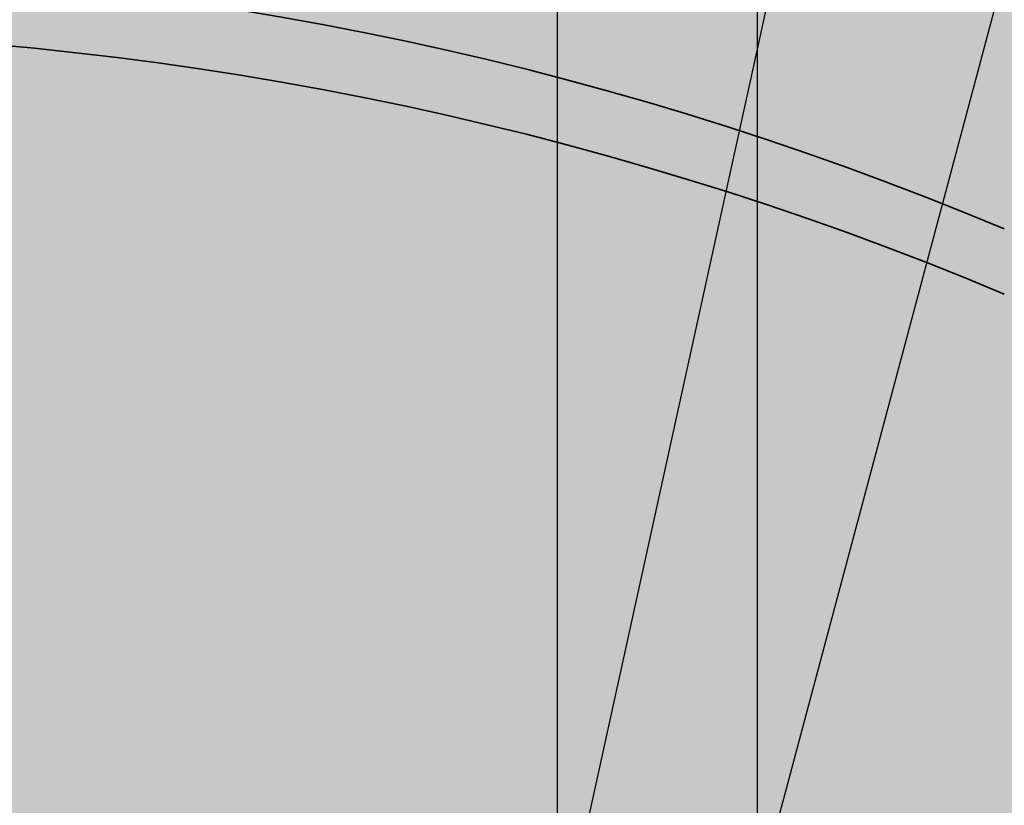
# Model space of a CAD drawing. Units: millimetres. Extents: x 130 to 1021, y 147 to 699.
# Tile 24 of 40: x 442 to 487, y 440 to 477. Entities that reach past the tile are written whole.
import ezdxf

# ---------------------------------------------------------------- set-up
doc = ezdxf.new("R2010")
doc.units = ezdxf.units.MM
doc.header["$MEASUREMENT"] = 0
for name, color, linetype, lineweight in [('A-ANNO-DIMS', 2, 'Continuous', 18), ('A-ELEV', 7, 'Continuous', 35), ('A-ELEV-PATT', 9, 'Continuous', 13)]:
    doc.layers.add(name, color=color, linetype=linetype, lineweight=lineweight)
doc.styles.get("Standard").update_dxf_attribs({"font": 'arial.ttf'})
doc.dimstyles.get("Standard").update_dxf_attribs({"dimtxt": 20, "dimasz": 10, "dimexe": 10, "dimexo": 10, "dimgap": 5, "dimtad": 0, "dimtih": 1, "dimtoh": 1, "dimdec": 0, "dimzin": 0, "dimdsep": 46, "dimtxsty": 'Standard', "dimcen": 5, "dimadec": 0, "dimazin": 0, "dimtfac": 1, "dimtdec": 0, "dimtofl": 0, "dimtmove": 0, "dimatfit": 3, "dimfxl": 1, "dimtolj": 1, "dimtzin": 0, "dimarcsym": 0})

# ---------------------------------------------------------------- blocks, each defined once
blk = doc.blocks.new('*D11')
at = {"layer": 'A-ANNO-DIMS', "color": 0, "lineweight": -2, "transparency": 16777216}
for p, q in [((737.374, 648.699), (737.374, 149.739)), ((299.374, 566.947), (299.374, 149.739)), ((309.374, 159.739), (490.857, 159.739)), ((727.374, 159.739), (545.891, 159.739))]:
    blk.add_line(p, q, dxfattribs=at)
at = {"layer": 'A-ANNO-DIMS', "color": 0, "transparency": 16777216}
for points in [[(309.374, 161.406), (309.374, 158.073), (299.374, 159.739)], [(727.374, 161.406), (727.374, 158.073), (737.374, 159.739)]]:
    blk.add_solid(points, dxfattribs=at)
at = {"layer": 'Defpoints', "color": 0, "transparency": 16777216}
for p in [(737.374, 658.699), (299.374, 576.947), (737.374, 159.739)]:
    blk.add_point(p, dxfattribs=at)
at = {"layer": 'A-ANNO-DIMS', "color": 0, "transparency": 16777216, "insert": (518.374, 159.739), "char_height": 20, "attachment_point": 5}
blk.add_mtext('\\A1;438', dxfattribs=at)
blk = doc.blocks.new('*D12')
at = {"layer": 'A-ANNO-DIMS', "color": 0, "lineweight": -2, "transparency": 16777216}
for p, q in [((477.374, 661.947), (265.074, 661.947)), ((275.074, 651.947), (275.074, 438.205)), ((275.074, 194.039), (275.074, 407.782)), ((357.163, 184.039), (265.074, 184.039))]:
    blk.add_line(p, q, dxfattribs=at)
at = {"layer": 'A-ANNO-DIMS', "color": 0, "transparency": 16777216}
for points in [[(273.407, 651.947), (276.74, 651.947), (275.074, 661.947)], [(273.407, 194.039), (276.74, 194.039), (275.074, 184.039)]]:
    blk.add_solid(points, dxfattribs=at)
at = {"layer": 'Defpoints', "color": 0, "transparency": 16777216}
for p in [(275.074, 661.947), (487.374, 661.947), (367.163, 184.039)]:
    blk.add_point(p, dxfattribs=at)
at = {"layer": 'A-ANNO-DIMS', "color": 0, "transparency": 16777216, "insert": (275.074, 422.993), "char_height": 20, "attachment_point": 5}
blk.add_mtext('\\A1;477.9', dxfattribs=at)
blk = doc.blocks.new('*D16')
at = {"layer": 'A-ANNO-DIMS', "color": 0, "lineweight": -2, "transparency": 16777216}
for p, q in [((357.941, 411.947), (357.941, 696.247)), ((363.922, 579.884), (363.922, 696.247)), ((347.941, 686.247), (337.941, 686.247)), ((373.922, 686.247), (383.922, 686.247))]:
    blk.add_line(p, q, dxfattribs=at)
at = {"layer": 'A-ANNO-DIMS', "color": 0, "transparency": 16777216}
for points in [[(347.941, 687.914), (347.941, 684.581), (357.941, 686.247)], [(373.922, 687.914), (373.922, 684.581), (363.922, 686.247)]]:
    blk.add_solid(points, dxfattribs=at)
at = {"layer": 'Defpoints', "color": 0, "transparency": 16777216}
for p in [(363.922, 686.247), (363.922, 569.884), (357.941, 401.947)]:
    blk.add_point(p, dxfattribs=at)
at = {"layer": 'A-ANNO-DIMS', "color": 0, "transparency": 16777216, "insert": (420.737, 686.247), "char_height": 20, "attachment_point": 5}
blk.add_mtext('\\A1;5.981', dxfattribs=at)
blk = doc.blocks.new('*D18')
at = {"layer": 'A-ANNO-DIMS', "color": 0, "lineweight": -2, "transparency": 16777216}
for p, q in [((375.85, 490.216), (375.85, 696.247)), ((382.374, 388.947), (382.374, 696.247)), ((365.85, 686.247), (355.85, 686.247)), ((392.374, 686.247), (402.374, 686.247))]:
    blk.add_line(p, q, dxfattribs=at)
at = {"layer": 'A-ANNO-DIMS', "color": 0, "transparency": 16777216}
for points in [[(365.85, 687.914), (365.85, 684.581), (375.85, 686.247)], [(392.374, 687.914), (392.374, 684.581), (382.374, 686.247)]]:
    blk.add_solid(points, dxfattribs=at)
at = {"layer": 'Defpoints', "color": 0, "transparency": 16777216}
for p in [(382.374, 686.247), (375.85, 480.216), (382.374, 378.947)]:
    blk.add_point(p, dxfattribs=at)
at = {"layer": 'A-ANNO-DIMS', "color": 0, "transparency": 16777216, "insert": (441.132, 686.247), "char_height": 20, "attachment_point": 5}
blk.add_mtext('\\A1;6.524', dxfattribs=at)
blk = doc.blocks.new('*D19')
at = {"layer": 'A-ANNO-DIMS', "color": 0, "lineweight": -2, "transparency": 16777216}
for p, q in [((382.374, 388.947), (382.374, 696.247)), ((414.652, 510.881), (414.652, 696.247)), ((392.374, 686.247), (404.652, 686.247)), ((414.652, 686.247), (424.652, 686.247))]:
    blk.add_line(p, q, dxfattribs=at)
at = {"layer": 'A-ANNO-DIMS', "color": 0, "transparency": 16777216}
for points in [[(392.374, 687.914), (392.374, 684.581), (382.374, 686.247)], [(404.652, 687.914), (404.652, 684.581), (414.652, 686.247)]]:
    blk.add_solid(points, dxfattribs=at)
at = {"layer": 'Defpoints', "color": 0, "transparency": 16777216}
for p in [(414.652, 686.247), (414.652, 500.881), (382.374, 378.947)]:
    blk.add_point(p, dxfattribs=at)
at = {"layer": 'A-ANNO-DIMS', "color": 0, "transparency": 16777216, "insert": (463.411, 686.247), "char_height": 20, "attachment_point": 5}
blk.add_mtext('\\A1;32.28', dxfattribs=at)
blk = doc.blocks.new('*D20')
at = {"layer": 'A-ANNO-DIMS', "color": 0, "lineweight": -2, "transparency": 16777216}
for p, q in [((414.652, 510.881), (414.652, 696.247)), ((432.374, 388.947), (432.374, 696.247)), ((404.652, 686.247), (394.652, 686.247)), ((442.374, 686.247), (452.374, 686.247))]:
    blk.add_line(p, q, dxfattribs=at)
at = {"layer": 'A-ANNO-DIMS', "color": 0, "transparency": 16777216}
for points in [[(404.652, 687.914), (404.652, 684.581), (414.652, 686.247)], [(442.374, 687.914), (442.374, 684.581), (432.374, 686.247)]]:
    blk.add_solid(points, dxfattribs=at)
at = {"layer": 'Defpoints', "color": 0, "transparency": 16777216}
for p in [(432.374, 686.247), (414.652, 500.881), (432.374, 378.947)]:
    blk.add_point(p, dxfattribs=at)
at = {"layer": 'A-ANNO-DIMS', "color": 0, "transparency": 16777216, "insert": (490.075, 686.247), "char_height": 20, "attachment_point": 5}
blk.add_mtext('\\A1;17.72', dxfattribs=at)
blk = doc.blocks.new('*D21')
at = {"layer": 'A-ANNO-DIMS', "color": 0, "lineweight": -2, "transparency": 16777216}
for p, q in [((432.374, 388.947), (432.374, 696.247)), ((447.374, 656.947), (447.374, 696.247)), ((422.374, 686.247), (412.374, 686.247)), ((457.374, 686.247), (467.374, 686.247))]:
    blk.add_line(p, q, dxfattribs=at)
at = {"layer": 'A-ANNO-DIMS', "color": 0, "transparency": 16777216}
for points in [[(422.374, 687.914), (422.374, 684.581), (432.374, 686.247)], [(457.374, 687.914), (457.374, 684.581), (447.374, 686.247)]]:
    blk.add_solid(points, dxfattribs=at)
at = {"layer": 'Defpoints', "color": 0, "transparency": 16777216}
for p in [(447.374, 686.247), (447.374, 646.947), (432.374, 378.947)]:
    blk.add_point(p, dxfattribs=at)
at = {"layer": 'A-ANNO-DIMS', "color": 0, "transparency": 16777216, "insert": (485.832, 686.247), "char_height": 20, "attachment_point": 5}
blk.add_mtext('\\A1;15', dxfattribs=at)
blk = doc.blocks.new('*D22')
at = {"layer": 'A-ANNO-DIMS', "color": 0, "lineweight": -2, "transparency": 16777216}
for p, q in [((447.374, 656.947), (447.374, 696.247)), ((466.767, 403.947), (466.767, 696.247)), ((437.374, 686.247), (427.374, 686.247)), ((476.767, 686.247), (486.767, 686.247))]:
    blk.add_line(p, q, dxfattribs=at)
at = {"layer": 'A-ANNO-DIMS', "color": 0, "transparency": 16777216}
for points in [[(437.374, 687.914), (437.374, 684.581), (447.374, 686.247)], [(476.767, 687.914), (476.767, 684.581), (466.767, 686.247)]]:
    blk.add_solid(points, dxfattribs=at)
at = {"layer": 'Defpoints', "color": 0, "transparency": 16777216}
for p in [(466.767, 686.247), (447.374, 646.947), (466.767, 393.947)]:
    blk.add_point(p, dxfattribs=at)
at = {"layer": 'A-ANNO-DIMS', "color": 0, "transparency": 16777216, "insert": (532.34, 686.247), "char_height": 20, "attachment_point": 5}
blk.add_mtext('\\A1;19.393', dxfattribs=at)
blk = doc.blocks.new('*D23')
at = {"layer": 'A-ANNO-DIMS', "color": 0, "lineweight": -2, "transparency": 16777216}
for p, q in [((466.767, 403.947), (466.767, 696.247)), ((475.988, 209.039), (475.988, 696.247)), ((456.767, 686.247), (446.767, 686.247)), ((485.988, 686.247), (495.988, 686.247))]:
    blk.add_line(p, q, dxfattribs=at)
at = {"layer": 'A-ANNO-DIMS', "color": 0, "transparency": 16777216}
for points in [[(456.767, 687.914), (456.767, 684.581), (466.767, 686.247)], [(485.988, 687.914), (485.988, 684.581), (475.988, 686.247)]]:
    blk.add_solid(points, dxfattribs=at)
at = {"layer": 'Defpoints', "color": 0, "transparency": 16777216}
for p in [(475.988, 686.247), (466.767, 393.947), (475.988, 199.039)]:
    blk.add_point(p, dxfattribs=at)
at = {"layer": 'A-ANNO-DIMS', "color": 0, "transparency": 16777216, "insert": (534.631, 686.247), "char_height": 20, "attachment_point": 5}
blk.add_mtext('\\A1;9.222', dxfattribs=at)
blk = doc.blocks.new('*D24')
at = {"layer": 'A-ANNO-DIMS', "color": 0, "lineweight": -2, "transparency": 16777216}
for p, q in [((475.988, 209.039), (475.988, 696.247)), ((487.374, 671.947), (487.374, 696.247)), ((465.988, 686.247), (455.988, 686.247)), ((497.374, 686.247), (507.374, 686.247))]:
    blk.add_line(p, q, dxfattribs=at)
at = {"layer": 'A-ANNO-DIMS', "color": 0, "transparency": 16777216}
for points in [[(465.988, 687.914), (465.988, 684.581), (475.988, 686.247)], [(497.374, 687.914), (497.374, 684.581), (487.374, 686.247)]]:
    blk.add_solid(points, dxfattribs=at)
at = {"layer": 'Defpoints', "color": 0, "transparency": 16777216}
for p in [(487.374, 686.247), (487.374, 661.947), (475.988, 199.039)]:
    blk.add_point(p, dxfattribs=at)
at = {"layer": 'A-ANNO-DIMS', "color": 0, "transparency": 16777216, "insert": (553.022, 686.247), "char_height": 20, "attachment_point": 5}
blk.add_mtext('\\A1;11.385', dxfattribs=at)
blk = doc.blocks.new('*D64')
at = {"layer": 'A-ANNO-DIMS', "color": 0, "lineweight": -2, "transparency": 16777216}
for p, q in [((502.049, 450.926), (502.049, 460.926)), ((497.049, 455.926), (507.049, 455.926)), ((363.96, 263.061), (409.922, 327.255)), ((353.96, 263.061), (363.96, 263.061))]:
    blk.add_line(p, q, dxfattribs=at)
at = {"layer": 'A-ANNO-DIMS', "color": 0, "transparency": 16777216}
blk.add_solid([(408.567, 328.225), (411.277, 326.284), (415.743, 335.385)], dxfattribs=at)
at = {"layer": 'Defpoints', "color": 0, "transparency": 16777216}
for p in [(502.049, 455.926), (415.743, 335.385)]:
    blk.add_point(p, dxfattribs=at)
at = {"layer": 'A-ANNO-DIMS', "color": 0, "transparency": 16777216, "insert": (297.8, 263.061), "char_height": 20, "attachment_point": 5}
blk.add_mtext('\\A1;R148.25', dxfattribs=at)
blk = doc.blocks.new('*D65')
at = {"layer": 'A-ANNO-DIMS', "color": 0, "lineweight": -2, "transparency": 16777216}
for p, q in [((495.463, 509.127), (472.508, 423.108)), ((505.463, 509.127), (495.463, 509.127)), ((427.374, 248.979), (427.374, 258.979)), ((422.374, 253.979), (432.374, 253.979))]:
    blk.add_line(p, q, dxfattribs=at)
at = {"layer": 'A-ANNO-DIMS', "color": 0, "transparency": 16777216}
blk.add_solid([(470.898, 423.538), (474.118, 422.679), (469.93, 413.447)], dxfattribs=at)
at = {"layer": 'Defpoints', "color": 0, "transparency": 16777216}
for p in [(469.93, 413.447), (427.374, 253.979)]:
    blk.add_point(p, dxfattribs=at)
at = {"layer": 'A-ANNO-DIMS', "color": 0, "transparency": 16777216, "insert": (561.623, 509.127), "char_height": 20, "attachment_point": 5}
blk.add_mtext('\\A1;R165.05', dxfattribs=at)
blk = doc.blocks.new('*D67')
at = {"layer": 'A-ANNO-DIMS', "color": 0, "lineweight": -2, "transparency": 16777216}
for p, q in [((479.756, 492.431), (462.144, 412.223)), ((489.756, 492.431), (479.756, 492.431)), ((427.07, 247.496), (427.07, 257.496)), ((422.07, 252.496), (432.07, 252.496))]:
    blk.add_line(p, q, dxfattribs=at)
at = {"layer": 'A-ANNO-DIMS', "color": 0, "transparency": 16777216}
blk.add_solid([(460.516, 412.58), (463.772, 411.865), (459.999, 402.455)], dxfattribs=at)
at = {"layer": 'Defpoints', "color": 0, "transparency": 16777216}
for p in [(459.999, 402.455), (427.07, 252.496)]:
    blk.add_point(p, dxfattribs=at)
at = {"layer": 'A-ANNO-DIMS', "color": 0, "transparency": 16777216, "insert": (545.841, 492.431), "char_height": 20, "attachment_point": 5}
blk.add_mtext('\\A1;R153.53', dxfattribs=at)
blk = doc.blocks.new('*D69')
at = {"layer": 'A-ANNO-DIMS', "color": 0, "lineweight": -2, "transparency": 16777216}
for p, q in [((507.746, 572.261), (483.091, 501.813)), ((517.746, 572.261), (507.746, 572.261)), ((433.191, 354.23), (433.191, 364.23)), ((428.191, 359.23), (438.191, 359.23))]:
    blk.add_line(p, q, dxfattribs=at)
at = {"layer": 'A-ANNO-DIMS', "color": 0, "transparency": 16777216}
blk.add_solid([(481.518, 502.363), (484.664, 501.262), (479.788, 492.374)], dxfattribs=at)
at = {"layer": 'Defpoints', "color": 0, "transparency": 16777216}
for p in [(479.788, 492.374), (433.191, 359.23)]:
    blk.add_point(p, dxfattribs=at)
at = {"layer": 'A-ANNO-DIMS', "color": 0, "transparency": 16777216, "insert": (573.824, 572.261), "char_height": 20, "attachment_point": 5}
blk.add_mtext('\\A1;R141.06', dxfattribs=at)
blk = doc.blocks.new('*D71')
at = {"layer": 'A-ANNO-DIMS', "color": 0, "lineweight": -2, "transparency": 16777216}
for p, q in [((492.108, 581.609), (472.542, 512.666)), ((502.108, 581.609), (492.108, 581.609)), ((432.65, 367.109), (432.65, 377.109)), ((427.65, 372.109), (437.65, 372.109))]:
    blk.add_line(p, q, dxfattribs=at)
at = {"layer": 'A-ANNO-DIMS', "color": 0, "transparency": 16777216}
blk.add_solid([(470.938, 513.121), (474.145, 512.211), (469.812, 503.046)], dxfattribs=at)
at = {"layer": 'Defpoints', "color": 0, "transparency": 16777216}
for p in [(469.812, 503.046), (432.65, 372.109)]:
    blk.add_point(p, dxfattribs=at)
at = {"layer": 'A-ANNO-DIMS', "color": 0, "transparency": 16777216, "insert": (548.493, 581.609), "char_height": 20, "attachment_point": 5}
blk.add_mtext('\\A1;R136.1', dxfattribs=at)
blk = doc.blocks.new('*D72')
at = {"layer": 'A-ANNO-DIMS', "color": 0, "lineweight": -2, "transparency": 16777216}
for p, q in [((460.658, 573.64), (451.279, 503.49)), ((470.658, 573.64), (460.658, 573.64)), ((432.115, 355.142), (432.115, 365.142)), ((427.115, 360.142), (437.115, 360.142))]:
    blk.add_line(p, q, dxfattribs=at)
at = {"layer": 'A-ANNO-DIMS', "color": 0, "transparency": 16777216}
blk.add_solid([(449.628, 503.711), (452.931, 503.27), (449.954, 493.579)], dxfattribs=at)
at = {"layer": 'Defpoints', "color": 0, "transparency": 16777216}
for p in [(449.954, 493.579), (432.115, 360.142)]:
    blk.add_point(p, dxfattribs=at)
at = {"layer": 'A-ANNO-DIMS', "color": 0, "transparency": 16777216, "insert": (526.64, 573.64), "char_height": 20, "attachment_point": 5}
blk.add_mtext('\\A1;R134.62', dxfattribs=at)

msp = doc.modelspace()

# ---------------------------------------------------------------- hatches: boundary and pattern name
at = {"layer": 'A-ELEV-PATT'}
h = msp.add_hatch(color=256, dxfattribs=at)
h.dxf.hatch_style = 1
h.paths.add_polyline_path([(737.3738, 658.6988, 0.0135961), (632.4019, 661.9473), (607.3738, 661.9473), (487.3738, 661.9473), (487.3738, 649.9473), (607.3738, 649.9473), (632.3794, 649.9473, -0.0136841), (737.3738, 646.6784)])
h.paths.add_polyline_path([(732.3738, 643.9599, 0.0130529), (632.3738, 646.9473), (607.3738, 646.9473), (487.3738, 646.9473), (487.3738, 596.9473), (632.3738, 596.9473, -0.0130529), (732.3738, 593.9599)])
h.paths.add_polyline_path([(737.3738, 593.6732, 0.0137063), (632.3738, 596.9473), (487.3738, 596.9473), (487.3738, 586.9473), (632.355, 586.9473, -0.0137808), (737.3738, 583.6559)])
h.paths.add_polyline_path([(447.3738, 646.9473), (307.3738, 646.9473), (302.3738, 646.9473), (302.3738, 634.9473), (447.3738, 634.9473)])
h.paths.add_polyline_path([(447.3738, 631.9473), (307.3738, 631.9473), (307.3738, 586.9473), (447.3738, 586.9473)])
h.paths.add_polyline_path([(447.3738, 586.9473), (307.3738, 586.9473), (302.3738, 586.9473), (302.3738, 576.9473), (447.3738, 576.9473)])
h.paths.add_polyline_path([(447.3738, 573.9473), (367.3738, 573.9473), (367.3738, 539.9473), (447.3738, 539.9473)])
h.paths.add_polyline_path([(447.3738, 537.9473), (367.3738, 537.9473), (367.3738, 507.9473), (400.392, 507.4253, -0.001728), (401.3281, 507.6451, -0.5220025), (425.6117, 511.0391, -0.0391849), (447.3738, 510.4359), (447.3738, 510.7883)])
h.paths.add_polyline_path([(394.7238, 505.9473), (367.3738, 505.9473), (367.3738, 476.9473, -0.0146512), (375.8501, 480.2159), (376.1506, 499.2266, -0.0355419)])
h.paths.add_polyline_path([(632.3738, 583.9473), (552.3738, 583.9473), (552.3738, 550.9473), (632.3738, 550.9473)])
h.paths.add_polyline_path([(632.3738, 548.9473), (552.3738, 548.9473), (552.3738, 515.9473), (632.3738, 515.9473)])
h.paths.add_polyline_path([(632.3738, 513.9473), (552.3738, 513.9473), (552.3738, 476.9473), (632.3738, 476.9473)])
h.paths.add_polyline_path([(737.3738, 473.6903, 0.0136326), (632.3926, 476.9473), (552.3738, 476.9473), (487.3738, 476.9473), (487.3738, 466.9473), (632.3738, 466.9473, -0.0137063), (737.3738, 463.6732)])
h.paths.add_polyline_path([(732.3738, 460.9552, 0.0130741), (632.3681, 463.9473), (487.3738, 463.9473), (487.3738, 407.735, -0.0032286), (489.3544, 406.9473), (632.3926, 406.9473, -0.0129826), (732.3738, 403.9755)])
h.paths.add_polyline_path([(487.3738, 463.9473, 0.20133), (367.3738, 463.9473), (367.3738, 407.735, -0.1882031), (487.3738, 407.735)])
h.paths.add_polyline_path([(367.3738, 476.9473), (367.3738, 466.9473, -0.2013309), (487.3738, 466.9473), (487.3738, 476.9473, 0.20133)])
h.paths.add_polyline_path([(367.3738, 463.9473), (307.3738, 463.9473), (307.3738, 401.9473), (357.9413, 401.9473), (367.3738, 407.735)])
h.paths.add_polyline_path([(367.3738, 476.9473), (302.3738, 476.9473), (302.3738, 466.9473), (367.3738, 466.9473)])
h.paths.add_polyline_path([(632.8184, 366.9453), (552.3738, 366.9453), (552.3738, 393.9473), (632.8184, 393.9473)])
h.paths.add_polyline_path([(632.8184, 357.2114), (632.8184, 363.9453), (552.3738, 363.9453), (552.3738, 357.2114), (552.3738, 336.9453), (632.8184, 336.9453)])
h.paths.add_polyline_path([(632.8184, 333.9453), (552.3738, 333.9453), (552.3738, 306.9453), (632.8184, 306.9453)])
h.paths.add_polyline_path([(632.8184, 303.9453), (552.3738, 303.9453), (552.3738, 273.9473), (632.355, 273.9473, 0.0000608), (632.8184, 273.9491)])
h.paths.add_polyline_path([(737.3738, 403.6903, 0.0136326), (632.3926, 406.9473), (489.3544, 406.9473, 0.1915481), (367.3738, 407.735), (367.3738, 396.9473, -0.2013309), (487.3738, 396.9473), (632.3738, 396.9473, -0.0137063), (737.3738, 393.6732)])
h.paths.add_polyline_path([(357.9413, 401.9473), (307.3738, 401.9473), (307.3738, 391.9473), (357.9413, 391.9473)])
h.paths.add_polyline_path([(357.9413, 357.2114), (357.9413, 388.9473), (307.3738, 388.9473), (307.3738, 357.2114), (307.3738, 273.9473), (357.9413, 273.9473)])
h.paths.add_polyline_path([(732.3738, 263.93, -0.0130317), (632.3794, 260.9473), (466.7667, 260.9473), (466.7667, 240.9473), (469.8406, 236.978), (469.8406, 221.978), (472.9145, 218.0087), (472.9145, 213.9473), (607.3738, 213.9473), (732.3738, 213.9473)])
h.paths.add_polyline_path([(732.3738, 290.889), (722.479, 290.889), (722.479, 301.889), (732.3738, 301.889), (732.3738, 305.889), (722.479, 305.889), (722.479, 316.889), (732.3738, 316.889), (732.3738, 320.889), (722.479, 320.889), (722.479, 331.889), (732.3738, 331.889), (732.3738, 335.889), (722.479, 335.889), (722.479, 346.889), (732.3738, 346.889), (732.3738, 350.889), (722.479, 350.889), (722.479, 361.889), (732.3738, 361.889), (732.3738, 365.889), (722.479, 365.889), (722.479, 376.889), (732.3738, 376.889), (732.3738, 380.889), (722.479, 380.889), (722.479, 391.4848, 0.0005233), (718.479, 391.6843), (718.479, 380.889), (707.479, 380.889), (707.479, 392.1896, 0.0005231), (703.479, 392.3576), (703.479, 380.889), (692.479, 380.889), (692.479, 392.7765, 0.0005229), (688.479, 392.9131), (688.479, 380.889), (677.479, 380.889), (677.479, 393.2456, 0.0005228), (673.479, 393.3508), (673.479, 380.889), (662.479, 380.889), (662.479, 393.597, 0.0005227), (658.479, 393.6709), (658.479, 380.889), (647.479, 380.889), (647.479, 393.8308, 0.0005226), (643.479, 393.8732), (643.479, 380.889), (632.8184, 380.889), (632.8184, 376.889), (643.479, 376.889), (643.479, 365.889), (632.8184, 365.889), (632.8184, 361.889), (643.479, 361.889), (643.479, 350.889), (632.8184, 350.889), (632.8184, 346.889), (643.479, 346.889), (643.479, 335.889), (632.8184, 335.889), (632.8184, 331.889), (643.479, 331.889), (643.479, 320.889), (632.8184, 320.889), (632.8184, 316.889), (643.479, 316.889), (643.479, 305.889), (632.8184, 305.889), (632.8184, 301.889), (643.479, 301.889), (643.479, 290.889), (632.8184, 290.889), (632.8184, 286.889), (643.479, 286.889), (643.479, 274.0217, 0.0005246), (647.479, 274.0643), (647.479, 286.889), (658.479, 286.889), (658.479, 274.2248, 0.0005246), (662.479, 274.2989), (662.479, 286.889), (673.479, 286.889), (673.479, 274.546, 0.0005247), (677.479, 274.6516), (677.479, 286.889), (688.479, 286.889), (688.479, 274.9853, 0.0005248), (692.479, 275.1224), (692.479, 286.889), (703.479, 286.889), (703.479, 275.5429, 0.000525), (707.479, 275.7115), (707.479, 286.889), (718.479, 286.889), (718.479, 276.2187, 0.0005252), (722.479, 276.4189), (722.479, 286.889), (732.3738, 286.889)])
h.paths.add_polyline_path([(718.479, 290.889), (707.479, 290.889), (707.479, 301.889), (718.479, 301.889)], flags=16)
h.paths.add_polyline_path([(703.479, 290.889), (692.479, 290.889), (692.479, 301.889), (703.479, 301.889)], flags=16)
h.paths.add_polyline_path([(718.479, 305.889), (707.479, 305.889), (707.479, 316.889), (718.479, 316.889)], flags=16)
h.paths.add_polyline_path([(703.479, 305.889), (692.479, 305.889), (692.479, 316.889), (703.479, 316.889)], flags=16)
h.paths.add_polyline_path([(688.479, 290.889), (677.479, 290.889), (677.479, 301.889), (688.479, 301.889)], flags=16)
h.paths.add_polyline_path([(718.479, 320.889), (707.479, 320.889), (707.479, 331.889), (718.479, 331.889)], flags=16)
h.paths.add_polyline_path([(688.479, 305.889), (677.479, 305.889), (677.479, 316.889), (688.479, 316.889)], flags=16)
h.paths.add_polyline_path([(703.479, 320.889), (692.479, 320.889), (692.479, 331.889), (703.479, 331.889)], flags=16)
h.paths.add_polyline_path([(688.479, 320.889), (677.479, 320.889), (677.479, 331.889), (688.479, 331.889)], flags=16)
h.paths.add_polyline_path([(673.479, 290.889), (662.479, 290.889), (662.479, 301.889), (673.479, 301.889)], flags=16)
h.paths.add_polyline_path([(718.479, 335.889), (707.479, 335.889), (707.479, 346.889), (718.479, 346.889)], flags=16)
h.paths.add_polyline_path([(673.479, 305.889), (662.479, 305.889), (662.479, 316.889), (673.479, 316.889)], flags=16)
h.paths.add_polyline_path([(703.479, 335.889), (692.479, 335.889), (692.479, 346.889), (703.479, 346.889)], flags=16)
h.paths.add_polyline_path([(673.479, 320.889), (662.479, 320.889), (662.479, 331.889), (673.479, 331.889)], flags=16)
h.paths.add_polyline_path([(688.479, 335.889), (677.479, 335.889), (677.479, 346.889), (688.479, 346.889)], flags=16)
h.paths.add_polyline_path([(658.479, 290.889), (647.479, 290.889), (647.479, 301.889), (658.479, 301.889)], flags=16)
h.paths.add_polyline_path([(718.479, 350.889), (707.479, 350.889), (707.479, 361.889), (718.479, 361.889)], flags=16)
h.paths.add_polyline_path([(658.479, 305.889), (647.479, 305.889), (647.479, 316.889), (658.479, 316.889)], flags=16)
h.paths.add_polyline_path([(703.479, 350.889), (692.479, 350.889), (692.479, 361.889), (703.479, 361.889)], flags=16)
h.paths.add_polyline_path([(673.479, 335.889), (662.479, 335.889), (662.479, 346.889), (673.479, 346.889)], flags=16)
h.paths.add_polyline_path([(658.479, 320.889), (647.479, 320.889), (647.479, 331.889), (658.479, 331.889)], flags=16)
h.paths.add_polyline_path([(688.479, 350.889), (677.479, 350.889), (677.479, 361.889), (688.479, 361.889)], flags=16)
h.paths.add_polyline_path([(718.479, 365.889), (707.479, 365.889), (707.479, 376.889), (718.479, 376.889)], flags=16)
h.paths.add_polyline_path([(658.479, 335.889), (647.479, 335.889), (647.479, 346.889), (658.479, 346.889)], flags=16)
h.paths.add_polyline_path([(673.479, 350.889), (662.479, 350.889), (662.479, 361.889), (673.479, 361.889)], flags=16)
h.paths.add_polyline_path([(703.479, 365.889), (692.479, 365.889), (692.479, 376.889), (703.479, 376.889)], flags=16)
h.paths.add_polyline_path([(688.479, 365.889), (677.479, 365.889), (677.479, 376.889), (688.479, 376.889)], flags=16)
h.paths.add_polyline_path([(658.479, 350.889), (647.479, 350.889), (647.479, 361.889), (658.479, 361.889)], flags=16)
h.paths.add_polyline_path([(673.479, 365.889), (662.479, 365.889), (662.479, 376.889), (673.479, 376.889)], flags=16)
h.paths.add_polyline_path([(658.479, 365.889), (647.479, 365.889), (647.479, 376.889), (658.479, 376.889)], flags=16)
h.paths.add_polyline_path([(732.3738, 503.9786), (722.3392, 503.9786), (722.3392, 514.9786), (732.3738, 514.9786), (732.3738, 518.9786), (722.3392, 518.9786), (722.3392, 529.9786), (732.3738, 529.9786), (732.3738, 533.9786), (722.3392, 533.9786), (722.3392, 544.9786), (732.3738, 544.9786), (732.3738, 546.9473), (732.3738, 548.9786), (722.3392, 548.9786), (722.3392, 559.9786), (732.3738, 559.9786), (732.3738, 563.9786), (722.3392, 563.9786), (722.3392, 574.9786), (732.3738, 574.9786), (732.3738, 578.9786), (722.3392, 578.9786), (722.3392, 581.4789, 0.000526), (718.3392, 581.6791), (718.3392, 578.9786), (707.3392, 578.9786), (707.3392, 582.1863, 0.0005258), (703.3392, 582.355), (703.3392, 578.9786), (692.3392, 578.9786), (692.3392, 582.7752, 0.0005257), (688.3392, 582.9123), (688.3392, 578.9786), (677.3392, 578.9786), (677.3392, 583.2457, 0.0005255), (673.3392, 583.3512), (673.3392, 578.9786), (662.3392, 578.9786), (662.3392, 583.5978, 0.0005254), (658.3392, 583.6718), (658.3392, 578.9786), (647.3392, 578.9786), (647.3392, 583.8317, 0.0005254), (643.3392, 583.8741), (643.3392, 578.9786), (632.3738, 578.9786), (632.3738, 574.9786), (643.3392, 574.9786), (643.3392, 563.9786), (632.3738, 563.9786), (632.3738, 559.9786), (643.3392, 559.9786), (643.3392, 548.9786), (632.3738, 548.9786), (632.3738, 544.9786), (643.3392, 544.9786), (643.3392, 533.9786), (632.3738, 533.9786), (632.3738, 529.9786), (643.3392, 529.9786), (643.3392, 518.9786), (632.3738, 518.9786), (632.3738, 515.9473), (632.3738, 514.9786), (643.3392, 514.9786), (643.3392, 503.9786), (632.3738, 503.9786), (632.3738, 499.9786), (643.3392, 499.9786), (643.3392, 488.9786), (632.3738, 488.9786), (632.3738, 484.9786), (643.3392, 484.9786), (643.3392, 476.8751, -0.0005191), (647.3392, 476.8332), (647.3392, 484.9786), (658.3392, 484.9786), (658.3392, 476.6752, -0.0005192), (662.3392, 476.6022), (662.3392, 484.9786), (673.3392, 484.9786), (673.3392, 476.3585, -0.0005193), (677.3392, 476.2543), (677.3392, 484.9786), (688.3392, 484.9786), (688.3392, 475.9248, -0.0005194), (692.3392, 475.7894), (692.3392, 484.9786), (703.3392, 484.9786), (703.3392, 475.3741, -0.0005195), (707.3392, 475.2075), (707.3392, 484.9786), (718.3392, 484.9786), (718.3392, 474.7064, -0.0005197), (722.3392, 474.5086), (722.3392, 484.9786), (732.3738, 484.9786), (732.3738, 488.9786), (722.3392, 488.9786), (722.3392, 499.9786), (732.3738, 499.9786)])
h.paths.add_polyline_path([(718.3392, 503.9786), (707.3392, 503.9786), (707.3392, 514.9786), (718.3392, 514.9786)], flags=16)
h.paths.add_polyline_path([(718.3392, 499.9786), (718.3392, 488.9786), (707.3392, 488.9786), (707.3392, 499.9786)], flags=16)
h.paths.add_polyline_path([(718.3392, 518.9786), (707.3392, 518.9786), (707.3392, 529.9786), (718.3392, 529.9786)], flags=16)
h.paths.add_polyline_path([(703.3392, 503.9786), (692.3392, 503.9786), (692.3392, 514.9786), (703.3392, 514.9786)], flags=16)
h.paths.add_polyline_path([(703.3392, 499.9786), (703.3392, 488.9786), (692.3392, 488.9786), (692.3392, 499.9786)], flags=16)
h.paths.add_polyline_path([(703.3392, 518.9786), (692.3392, 518.9786), (692.3392, 529.9786), (703.3392, 529.9786)], flags=16)
h.paths.add_polyline_path([(718.3392, 533.9786), (707.3392, 533.9786), (707.3392, 544.9786), (718.3392, 544.9786)], flags=16)
h.paths.add_polyline_path([(688.3392, 503.9786), (677.3392, 503.9786), (677.3392, 514.9786), (688.3392, 514.9786)], flags=16)
h.paths.add_polyline_path([(688.3392, 499.9786), (688.3392, 488.9786), (677.3392, 488.9786), (677.3392, 499.9786)], flags=16)
h.paths.add_polyline_path([(703.3392, 533.9786), (692.3392, 533.9786), (692.3392, 544.9786), (703.3392, 544.9786)], flags=16)
h.paths.add_polyline_path([(688.3392, 518.9786), (677.3392, 518.9786), (677.3392, 529.9786), (688.3392, 529.9786)], flags=16)
h.paths.add_polyline_path([(688.3392, 533.9786), (677.3392, 533.9786), (677.3392, 544.9786), (688.3392, 544.9786)], flags=16)
h.paths.add_polyline_path([(718.3392, 548.9786), (707.3392, 548.9786), (707.3392, 559.9786), (718.3392, 559.9786)], flags=16)
h.paths.add_polyline_path([(673.3392, 503.9786), (662.3392, 503.9786), (662.3392, 514.9786), (673.3392, 514.9786)], flags=16)
h.paths.add_polyline_path([(673.3392, 499.9786), (673.3392, 488.9786), (662.3392, 488.9786), (662.3392, 499.9786)], flags=16)
h.paths.add_polyline_path([(703.3392, 548.9786), (692.3392, 548.9786), (692.3392, 559.9786), (703.3392, 559.9786)], flags=16)
h.paths.add_polyline_path([(673.3392, 518.9786), (662.3392, 518.9786), (662.3392, 529.9786), (673.3392, 529.9786)], flags=16)
h.paths.add_polyline_path([(688.3392, 548.9786), (677.3392, 548.9786), (677.3392, 559.9786), (688.3392, 559.9786)], flags=16)
h.paths.add_polyline_path([(673.3392, 533.9786), (662.3392, 533.9786), (662.3392, 544.9786), (673.3392, 544.9786)], flags=16)
h.paths.add_polyline_path([(718.3392, 563.9786), (707.3392, 563.9786), (707.3392, 574.9786), (718.3392, 574.9786)], flags=16)
h.paths.add_polyline_path([(658.3392, 503.9786), (647.3392, 503.9786), (647.3392, 514.9786), (658.3392, 514.9786)], flags=16)
h.paths.add_polyline_path([(658.3392, 499.9786), (658.3392, 488.9786), (647.3392, 488.9786), (647.3392, 499.9786)], flags=16)
h.paths.add_polyline_path([(703.3392, 563.9786), (692.3392, 563.9786), (692.3392, 574.9786), (703.3392, 574.9786)], flags=16)
h.paths.add_polyline_path([(658.3392, 518.9786), (647.3392, 518.9786), (647.3392, 529.9786), (658.3392, 529.9786)], flags=16)
h.paths.add_polyline_path([(673.3392, 548.9786), (662.3392, 548.9786), (662.3392, 559.9786), (673.3392, 559.9786)], flags=16)
h.paths.add_polyline_path([(688.3392, 563.9786), (677.3392, 563.9786), (677.3392, 574.9786), (688.3392, 574.9786)], flags=16)
h.paths.add_polyline_path([(658.3392, 533.9786), (647.3392, 533.9786), (647.3392, 544.9786), (658.3392, 544.9786)], flags=16)
h.paths.add_polyline_path([(673.3392, 563.9786), (662.3392, 563.9786), (662.3392, 574.9786), (673.3392, 574.9786)], flags=16)
h.paths.add_polyline_path([(658.3392, 548.9786), (647.3392, 548.9786), (647.3392, 559.9786), (658.3392, 559.9786)], flags=16)
h.paths.add_polyline_path([(658.3392, 563.9786), (647.3392, 563.9786), (647.3392, 574.9786), (658.3392, 574.9786)], flags=16)
h = msp.add_hatch(color=256, dxfattribs=at)
h.dxf.hatch_style = 1
h.paths.add_polyline_path([(447.3738, 576.9473), (302.3738, 576.9473), (302.3738, 573.9473), (447.3738, 573.9473)])
h.paths.add_polyline_path([(487.3738, 583.9473), (487.3738, 586.9473), (447.3738, 576.9473), (447.3738, 573.9473)])
h.paths.add_polyline_path([(632.355, 586.9473), (487.3738, 586.9473), (487.3738, 583.9473), (632.3738, 583.9473), (632.3738, 583.9472, -0.0138), (737.3738, 580.6507), (737.3738, 583.6559, 0.0137808)])
h.paths.add_polyline_path([(367.3738, 466.9473), (302.3738, 466.9473), (302.3738, 463.9473), (367.3738, 463.9473)])
h.paths.add_polyline_path([(487.3738, 463.9473), (487.3738, 466.9473, 0.2013309), (367.3738, 466.9473), (367.3738, 463.9473, -0.20133)])
h.paths.add_polyline_path([(632.3738, 466.9473), (487.3738, 466.9473), (487.3738, 463.9473), (632.3681, 463.9473, -0.0137285), (737.3738, 460.6681), (737.3738, 463.6732, 0.0137063)])
h.paths.add_polyline_path([(632.3738, 396.9473), (487.3738, 396.9473, 0.2013309), (367.3738, 396.9473), (367.3738, 393.9473, -0.2023717), (486.7667, 393.9473), (632.3681, 393.9473, -0.0137285), (737.3738, 390.6681), (737.3738, 393.6732, 0.0137063)])
h.paths.add_polyline_path([(357.9413, 391.9473), (307.3738, 391.9473), (307.3738, 388.9473), (357.9413, 388.9473)])
h.paths.add_polyline_path([(367.3738, 393.9473), (367.3738, 396.9473), (357.9413, 391.924), (357.9413, 388.9473), (358.058, 388.9473)])
h.paths.add_polyline_path([(737.3738, 264.2162), (737.3738, 267.2214, -0.0137063), (632.3738, 263.9473), (463.7667, 263.9473), (466.7667, 260.9473), (632.3794, 260.9473, 0.0136841)])
h.paths.add_polyline_path([(463.7667, 263.9473), (447.3738, 263.9473), (450.3738, 260.9473), (466.7667, 260.9473)])
h.paths.add_polyline_path([(447.3738, 263.9473), (432.3738, 263.9473), (432.3738, 260.9473), (450.3738, 260.9473)])
h.paths.add_polyline_path([(382.3738, 263.9473), (357.9413, 263.9473), (357.9413, 260.9473), (382.3738, 260.9473)])
h.paths.add_polyline_path([(357.9413, 263.9473), (307.3738, 263.9473), (307.3738, 260.9473), (357.9413, 260.9473)])

# ---------------------------------------------------------------- linework, layer by layer
at = {"layer": 'A-ELEV'}
for centre, radius, start, end in [((427.3738, 323.9788), 155.0484, 67.233534, 112.766466), ((427.3738, 320.9781), 155.049, 67.23363, 112.76637)]:
    msp.add_arc(centre, radius, start, end, dxfattribs=at)

# ---------------------------------------------------------------- dimensions: what is measured, and where the dimension line sits
at = {"layer": 'A-ANNO-DIMS'}
for base, p1, p2, override, picture, middle in [((363.922, 686.2473), (357.9413, 401.9473), (363.922, 569.884), {"dimdec": 3, "dimlfac": 1, "dimrnd": 0, "dimzin": 0, "dimdsep": 46, "dimlunit": 2}, '*D16', (420.7365, 686.2473)), ((382.3738, 686.2473), (375.8501, 480.2159), (382.3738, 378.9473), {"dimdec": 3, "dimlfac": 1, "dimrnd": 0, "dimzin": 0, "dimdsep": 46, "dimlunit": 2}, '*D18', (441.1323, 686.2473)), ((414.6525, 686.2473), (382.3738, 378.9473), (414.6525, 500.8811), {"dimdec": 2, "dimlfac": 1, "dimrnd": 0, "dimzin": 0, "dimdsep": 46, "dimlunit": 2}, '*D19', (463.411, 686.2473)), ((432.3738, 686.2473), (414.6525, 500.8811), (432.3738, 378.9473), {"dimdec": 2, "dimlfac": 1, "dimrnd": 0, "dimzin": 0, "dimdsep": 46, "dimlunit": 2}, '*D20', (490.075, 686.2473)), ((447.3738, 686.2473), (432.3738, 378.9473), (447.3738, 646.9473), {"dimdec": 0, "dimlfac": 1, "dimrnd": 0, "dimzin": 0, "dimdsep": 46, "dimlunit": 2}, '*D21', (485.8322, 686.2473)), ((466.7667, 686.2473), (447.3738, 646.9473), (466.7667, 393.9473), {"dimdec": 3, "dimlfac": 1, "dimrnd": 0, "dimzin": 0, "dimdsep": 46, "dimlunit": 2}, '*D22', (532.3397, 686.2473)), ((475.9885, 686.2473), (466.7667, 393.9473), (475.9885, 199.0395), {"dimdec": 3, "dimlfac": 1, "dimrnd": 0, "dimzin": 0, "dimdsep": 46, "dimlunit": 2}, '*D23', (534.631, 686.2473)), ((487.3738, 686.2473), (475.9885, 199.0395), (487.3738, 661.9473), {"dimdec": 3, "dimlfac": 1, "dimrnd": 0, "dimzin": 0, "dimdsep": 46, "dimlunit": 2}, '*D24', (553.0218, 686.2473)), ((737.3738, 159.7395), (299.3738, 576.9473), (737.3738, 658.6988), {"dimdec": 0, "dimlfac": 1, "dimrnd": 0, "dimzin": 0, "dimdsep": 46, "dimlunit": 2}, '*D11', (518.3738, 159.7395))]:
    dim = msp.add_linear_dim(base=base, p1=p1, p2=p2, dimstyle='Standard', override=override, dxfattribs=at)
    dim.commit()
    dim.dimension.update_dxf_attribs({"geometry": picture, "text_midpoint": middle})
dim = msp.add_linear_dim(base=(275.0738, 661.9473), p1=(367.163, 184.0395), p2=(487.3738, 661.9473), angle=90, dimstyle='Standard', override={"dimdec": 1, "dimlfac": 1, "dimrnd": 0, "dimzin": 0, "dimdsep": 46, "dimlunit": 2}, dxfattribs=at)
dim.commit()
dim.dimension.update_dxf_attribs({"geometry": '*D12', "text_midpoint": (275.0738, 422.9934)})
for center, mpoint, override, picture, middle in [((432.6505, 372.1087), (469.8116, 503.0461), {"dimdec": 1, "dimlfac": 1, "dimrnd": 0, "dimzin": 0, "dimdsep": 46, "dimlunit": 2}, '*D71', (548.493, 581.6085)), ((432.115, 360.1423), (449.9544, 493.5786), {"dimdec": 2, "dimlfac": 1, "dimrnd": 0, "dimzin": 0, "dimdsep": 46, "dimlunit": 2}, '*D72', (526.6403, 573.6404)), ((433.1906, 359.2304), (479.788, 492.3743), {"dimdec": 2, "dimlfac": 1, "dimrnd": 0, "dimzin": 0, "dimdsep": 46, "dimlunit": 2}, '*D69', (573.8242, 572.2606)), ((427.3738, 253.9788), (469.9297, 413.4465), {"dimdec": 2, "dimlfac": 1, "dimrnd": 0, "dimzin": 0, "dimdsep": 46, "dimlunit": 2}, '*D65', (561.6228, 509.1272)), ((427.0702, 252.4956), (459.999, 402.4554), {"dimdec": 2, "dimlfac": 1, "dimrnd": 0, "dimzin": 0, "dimdsep": 46, "dimlunit": 2}, '*D67', (545.8408, 492.4313)), ((502.0489, 455.9263), (415.7433, 335.3854), {"dimdec": 2, "dimlfac": 1, "dimrnd": 0, "dimzin": 0, "dimdsep": 46, "dimlunit": 2}, '*D64', (297.8003, 263.0608))]:
    dim = msp.add_radius_dim(center=center, mpoint=mpoint, dimstyle='Standard', override=override, dxfattribs=at)
    dim.commit()
    dim.dimension.update_dxf_attribs({"geometry": picture, "text_midpoint": middle, "dimtype": 164})

doc.saveas('drawing.dxf')
